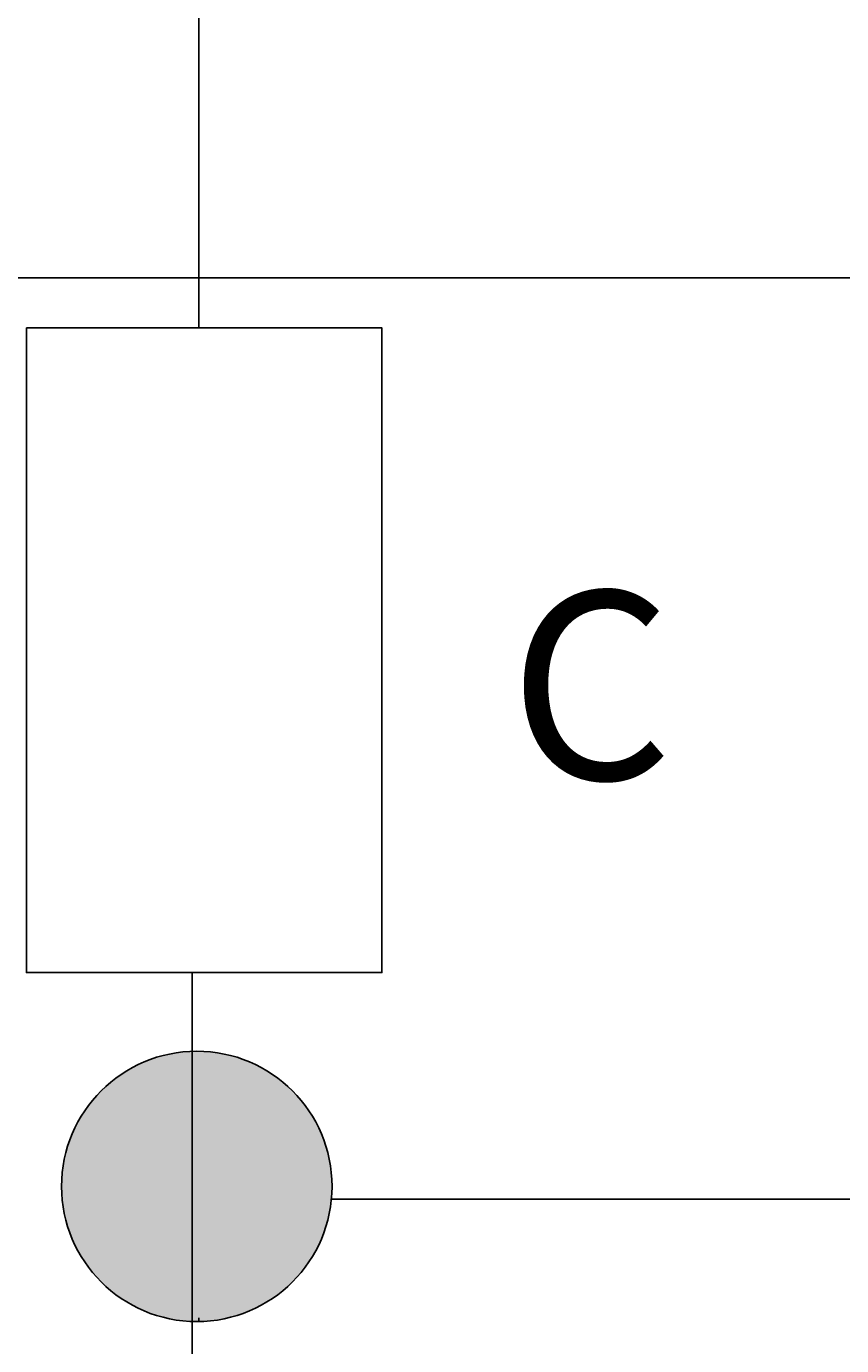
# Model space of a CAD drawing. Units: inches. Extents: x 35362 to 73946, y 43607 to 67532.
# Tile 134 of 134: x 68321 to 69277, y 57027 to 58575. Entities that reach past the tile are written whole.
import ezdxf

# ---------------------------------------------------------------- set-up
doc = ezdxf.new("R2010")
doc.units = ezdxf.units.IN
doc.header["$MEASUREMENT"] = 0
for name, color, linetype, lineweight in [('A-ANNO-DIMS', 2, 'Continuous', 18), ('E-ANNO-TEXT', 5, 'Continuous', 18), ('E-SYMB', 1, 'Continuous', 25), ('E-SYMB-PATT', 1, 'Continuous', 13), ('E-WIRE', 3, 'Continuous', 25)]:
    doc.layers.add(name, color=color, linetype=linetype, lineweight=lineweight)
doc.styles.get("Standard").update_dxf_attribs({"font": 'arial.ttf'})
doc.dimstyles.get("Standard").update_dxf_attribs({"dimtxt": 0.18, "dimasz": 0.18, "dimexe": 0.18, "dimexo": 0.0625, "dimgap": 0.09, "dimtad": 0, "dimtih": 1, "dimtoh": 1, "dimdec": 4, "dimzin": 0, "dimdsep": 46, "dimtxsty": 'Standard', "dimcen": 0.09, "dimadec": 0, "dimazin": 0, "dimtfac": 1, "dimtdec": 4, "dimtofl": 0, "dimtmove": 0, "dimatfit": 3, "dimfxl": 1, "dimtolj": 1, "dimtzin": 0, "dimarcsym": 0})

# ---------------------------------------------------------------- blocks, each defined once
blk = doc.blocks.new('*D8')
at = {"layer": 'A-ANNO-DIMS', "color": 0, "lineweight": -2, "transparency": 16777216}
for p, q in [((66271.28651900003, 65771.51172800003), (73945.82566600003, 65771.51172800003)), ((73945.64566600005, 65771.33172800003), (73945.64566600005, 59737.03093663782)), ((73945.64566600005, 53702.36633900002), (73945.64566600005, 59736.66713036224)), ((72185.70816600003, 53702.18633900003), (73945.82566600003, 53702.18633900003))]:
    blk.add_line(p, q, dxfattribs=at)
at = {"layer": 'A-ANNO-DIMS', "color": 0, "transparency": 16777216}
for points in [[(73945.61566600006, 65771.33172800003), (73945.67566600005, 65771.33172800003), (73945.64566600005, 65771.51172800003)], [(73945.61566600006, 53702.36633900002), (73945.67566600005, 53702.36633900002), (73945.64566600005, 53702.18633900003)]]:
    blk.add_solid(points, dxfattribs=at)
at = {"layer": 'Defpoints', "color": 0, "transparency": 16777216}
for p in [(66271.22401900003, 65771.51172800003), (73945.64566600005, 65771.51172800003), (72185.64566600003, 53702.18633900003)]:
    blk.add_point(p, dxfattribs=at)
at = {"layer": 'A-ANNO-DIMS', "color": 0, "transparency": 16777216, "insert": (73945.64566600005, 59736.84903349999), "char_height": 0.18, "attachment_point": 5}
blk.add_mtext('\\A1;12069', dxfattribs=at)
blk = doc.blocks.new('*D10')
at = {"layer": 'A-ANNO-DIMS', "color": 0, "lineweight": -2, "transparency": 16777216}
for p, q in [((61240.96983600002, 59185.14395700003), (73945.82566600003, 59185.14395700003)), ((73945.64566600005, 59184.96395700003), (73945.64566600005, 56268.51827402935)), ((73945.64566600005, 53351.70866200003), (73945.64566600005, 56268.1543449707)), ((61240.96983600002, 53351.52866200003), (73945.82566600003, 53351.52866200003))]:
    blk.add_line(p, q, dxfattribs=at)
at = {"layer": 'A-ANNO-DIMS', "color": 0, "transparency": 16777216}
for points in [[(73945.61566600006, 59184.96395700003), (73945.67566600005, 59184.96395700003), (73945.64566600005, 59185.14395700003)], [(73945.61566600006, 53351.70866200003), (73945.67566600005, 53351.70866200003), (73945.64566600005, 53351.52866200003)]]:
    blk.add_solid(points, dxfattribs=at)
at = {"layer": 'Defpoints', "color": 0, "transparency": 16777216}
for p in [(61240.90733600002, 59185.14395700003), (61240.90733600002, 53351.52866200003), (73945.64566600005, 53351.52866200003)]:
    blk.add_point(p, dxfattribs=at)
at = {"layer": 'A-ANNO-DIMS', "color": 0, "transparency": 16777216, "insert": (73945.64566600005, 56268.33630949999), "char_height": 0.18, "attachment_point": 5}
blk.add_mtext('\\A1;5834', dxfattribs=at)
blk = doc.blocks.new('*D47')
at = {"layer": 'A-ANNO-DIMS', "color": 0, "lineweight": -2, "transparency": 16777216}
for p, q in [((50339.58680000003, 58279.98849500002), (73945.82566600003, 58279.98849500002)), ((73945.64566600005, 58279.80849500002), (73945.64566600005, 57564.17141502935)), ((73945.64566600005, 56848.17040600003), (73945.64566600005, 57563.80748597069)), ((50339.58680000003, 56847.99040600003), (73945.82566600003, 56847.99040600003))]:
    blk.add_line(p, q, dxfattribs=at)
at = {"layer": 'A-ANNO-DIMS', "color": 0, "transparency": 16777216}
for points in [[(73945.61566600006, 58279.80849500002), (73945.67566600005, 58279.80849500002), (73945.64566600005, 58279.98849500002)], [(73945.61566600006, 56848.17040600003), (73945.67566600005, 56848.17040600003), (73945.64566600005, 56847.99040600003)]]:
    blk.add_solid(points, dxfattribs=at)
at = {"layer": 'Defpoints', "color": 0, "transparency": 16777216}
for p in [(50339.52430000002, 58279.98849500002), (50339.52430000002, 56847.99040600003), (73945.64566600005, 56847.99040600003)]:
    blk.add_point(p, dxfattribs=at)
at = {"layer": 'A-ANNO-DIMS', "color": 0, "transparency": 16777216, "insert": (73945.64566600005, 57563.98945049999), "char_height": 0.18, "attachment_point": 5}
blk.add_mtext('\\A1;1432.0', dxfattribs=at)

msp = doc.modelspace()

# ---------------------------------------------------------------- hatches: boundary and pattern name
at = {"layer": 'E-SYMB-PATT'}
h = msp.add_hatch(color=256, dxfattribs=at)
h.dxf.hatch_style = 1
h.paths.add_polyline_path([(68522.99328781641, 57372.21445361012, 0.4183931940818975), (68362.12749647925, 57213.62466823159, 0.4183931940818975), (68522.99328781641, 57055.03488285305)])
h.paths.add_polyline_path([(68522.99328781641, 57372.21445361012), (68522.99328781641, 57055.03488285305, 0.4100462469397049), (68679.33926925441, 57213.62466823159, 0.4100462469397049)])

# ---------------------------------------------------------------- linework, layer by layer
at = {"layer": 'E-SYMB'}
for p, q in [((68522.99328781641, 58468.38124608586), (68522.99328781641, 58221.08203096781)), ((68515.4609857722, 57464.46373729305), (68515.4609857722, 57372.14289754818)), ((68515.4609857722, 57372.14289754818), (68515.4609857722, 56943.54211886489)), ((68518.41798978415, 57372.21365319481), (68518.41798978415, 57371.52742993376)), ((68522.99328781641, 57059.50602833795), (68522.99328781641, 57055.03488285305))]:
    msp.add_line(p, q, dxfattribs=at)
msp.add_lwpolyline([(68320.87076221016, 58221.08203096781), (68737.80188109005, 58221.08203096781), (68737.80188109005, 57464.46373729305), (68320.87076221016, 57464.46373729305)], close=True, dxfattribs=at)
msp.add_circle((68520.73338286683, 57213.62466823159), 158.6058863875805, dxfattribs=at)
at = {"layer": 'E-WIRE'}
for p, q in [((68522.99328781641, 58468.38124608586), (68522.99328781641, 59095.61234402943)), ((68678.61631230469, 57198.49827444747), (69717.45127656069, 57198.49827444748))]:
    msp.add_line(p, q, dxfattribs=at)

# ---------------------------------------------------------------- texts
at = {"layer": 'E-ANNO-TEXT'}
msp.add_text('C', height=220.8659825270206, dxfattribs=at).set_placement((68886.85388514496, 57691.16137343028))

# ---------------------------------------------------------------- dimensions: what is measured, and where the dimension line sits
at = {"layer": 'A-ANNO-DIMS'}
for base, p1, p2, override, picture, middle in [((73945.64566600005, 65771.51172800003), (72185.645666, 53702.186339), (66271.224019, 65771.51172799998), {"dimdec": 0, "dimlfac": 1, "dimrnd": 0, "dimzin": 0, "dimdsep": 46, "dimlunit": 2}, '*D8', (73945.64566600005, 59736.84903349999)), ((73945.64566600005, 53351.52866200003), (61240.907336, 59185.14395699999), (61240.907336, 53351.52866199999), {"dimdec": 0, "dimlfac": 1, "dimrnd": 0, "dimzin": 0, "dimdsep": 46, "dimlunit": 2}, '*D10', (73945.64566600005, 56268.33630949999)), ((73945.64566600005, 56847.99040600003), (50339.5243, 58279.988495), (50339.5243, 56847.99040599999), {"dimdec": 1, "dimlfac": 1, "dimrnd": 0, "dimzin": 0, "dimdsep": 46, "dimlunit": 2}, '*D47', (73945.64566600005, 57563.98945049999))]:
    dim = msp.add_linear_dim(base=base, p1=p1, p2=p2, angle=90, dimstyle='Standard', override=override, dxfattribs=at)
    dim.commit()
    dim.dimension.update_dxf_attribs({"geometry": picture, "text_midpoint": middle})

doc.saveas('drawing.dxf')
